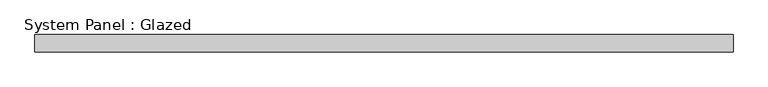
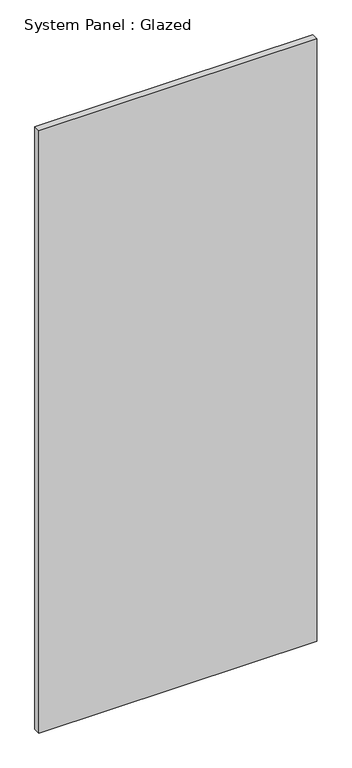
"""IFC4 building model written with IfcOpenShell, lengths in millimetres: plate geometry, System Panel : Glazed."""

from ifc_helpers import new_model, si_unit, origin, origin_with_axes, place, context, project, spatial, polyline, outline, extrude, source, transform, mapped, element, save


def system_panel_glazed_958d1135(model_context):
    return source(origin(), model_context, "Body", "SweptSolid", [
        extrude(outline(polyline([(511.175, 19.05), (-511.175, 19.05), (-511.175, 44.45), (511.175, 44.45), (511.175, 19.05)])), origin_with_axes(), (0.0, 0.0, 1.0), 2343.15),
    ])


if __name__ == "__main__":
    model = new_model("IFC4")
    model_context = context("Model", 3, world=origin())
    ifc_project = project(units=[si_unit("LENGTHUNIT", "METRE", prefix="MILLI")], contexts=[model_context])
    site = spatial("IfcSite", under=ifc_project)
    building = spatial("IfcBuilding", under=site)
    placement = place(None, origin())
    system_panel_glazed_shape = system_panel_glazed_958d1135(model_context)
    element("IfcPlate", 1, ObjectType="System Panel : Glazed", at=placement, inside=building, context=model_context, shape_type="MappedRepresentation", body=[
        mapped(system_panel_glazed_shape, transform((0.0, 0.0, 0.0), x_axis=(1.0, 0.0, 0.0), y_axis=(0.0, 1.0, 0.0), z_axis=(0.0, 0.0, 1.0))),
    ])
    save(model, "model.ifc")

# Revit data of these elements
# Type "System Panel : Glazed"
#   Construction Type Id = "GSP4R"
#   Analytic Construction = "1/8 in Pilkington single glazing"
#   Visual Light Transmittance = 0.9
#   Solar Heat Gain Coefficient = 0.86
#   Heat Transfer Coefficient (U) = 1.18115 BTU/(h·ft²·°F)
#   Define Thermal Properties by = 1
# Element 1 (IfcPlate, "System Panel : Glazed")
#   Materials on its faces: "Glass"
# Materials
#   "Glass": class "Glass", colour RGB 0 128 192, transparency 0.75, Description = "Soda Lime Glass", Cost = 0
